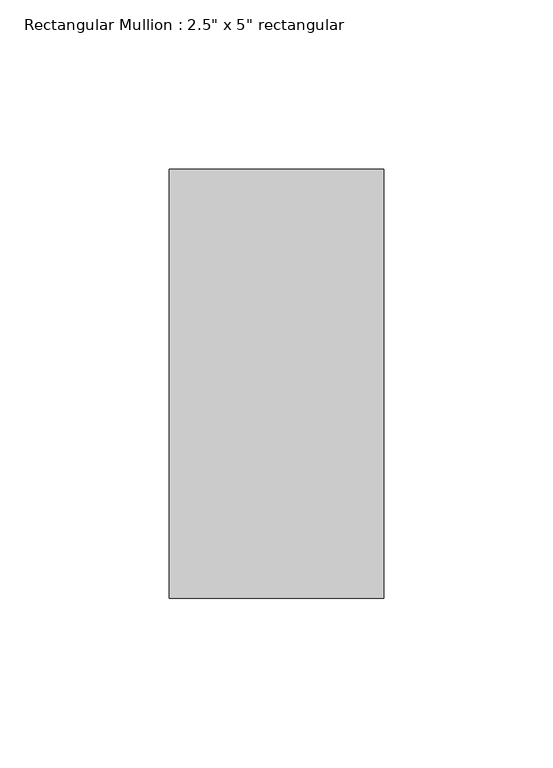
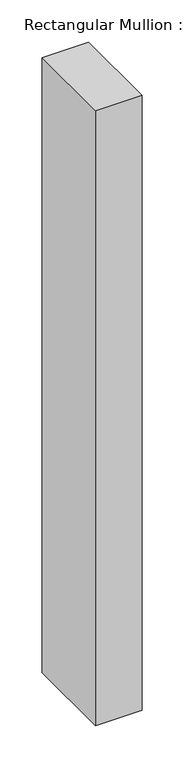
"""IFC4 building model written with IfcOpenShell, lengths in millimetres: member geometry."""

from ifc_helpers import new_model, si_unit, frame, origin, place, context, project, spatial, polyline, outline, extrude, source, transform, mapped, element, save


def member_9cf8e2d9(model_context):
    return source(origin(), model_context, "Body", "SweptSolid", [
        extrude(outline(polyline([(0.0, 63.5), (0.0, -63.5), (-63.5, -63.5), (-63.5, 63.5), (0.0, 63.5)])), frame((0.0, 0.0, -890.15), z_axis=(0.0, 0.0, 1.0), x_axis=(1.0, 0.0, 0.0)), (0.0, 0.0, 1.0), 890.15),
    ])


if __name__ == "__main__":
    model = new_model("IFC4")
    model_context = context("Model", 3, world=origin())
    ifc_project = project(units=[si_unit("LENGTHUNIT", "METRE", prefix="MILLI")], contexts=[model_context])
    site = spatial("IfcSite", under=ifc_project)
    building = spatial("IfcBuilding", under=site)
    placement = place(None, origin())
    member_shape = member_9cf8e2d9(model_context)
    element("IfcMember", 1, ObjectType="Rectangular Mullion : 2.5\" x 5\" rectangular", at=placement, inside=building, context=model_context, shape_type="MappedRepresentation", body=[
        mapped(member_shape, transform((0.0, 0.0, 0.0), x_axis=(1.0, 0.0, 0.0), y_axis=(0.0, 1.0, 0.0), z_axis=(0.0, 0.0, 1.0))),
    ])
    save(model, "model.ifc")

# Revit data of these elements
# Type "Rectangular Mullion : 2.5\" x 5\" rectangular"
#   built-in parameter 1007304 = 0.416667 (stored number, unit not read)
#   built-in parameter 1007301 = 0.104167 (stored number, unit not read)
#   built-in parameter 1007300 = 0.104167 (stored number, unit not read)
# Element 1 (IfcMember, "Rectangular Mullion : 2.5\" x 5\" rectangular")
#   Materials on its faces: "Damp-proofing"
# Materials
#   "Damp-proofing": class "Generic", colour RGB 127 127 127, transparency 0, Description = "Damp-proofing", Cost = 0
